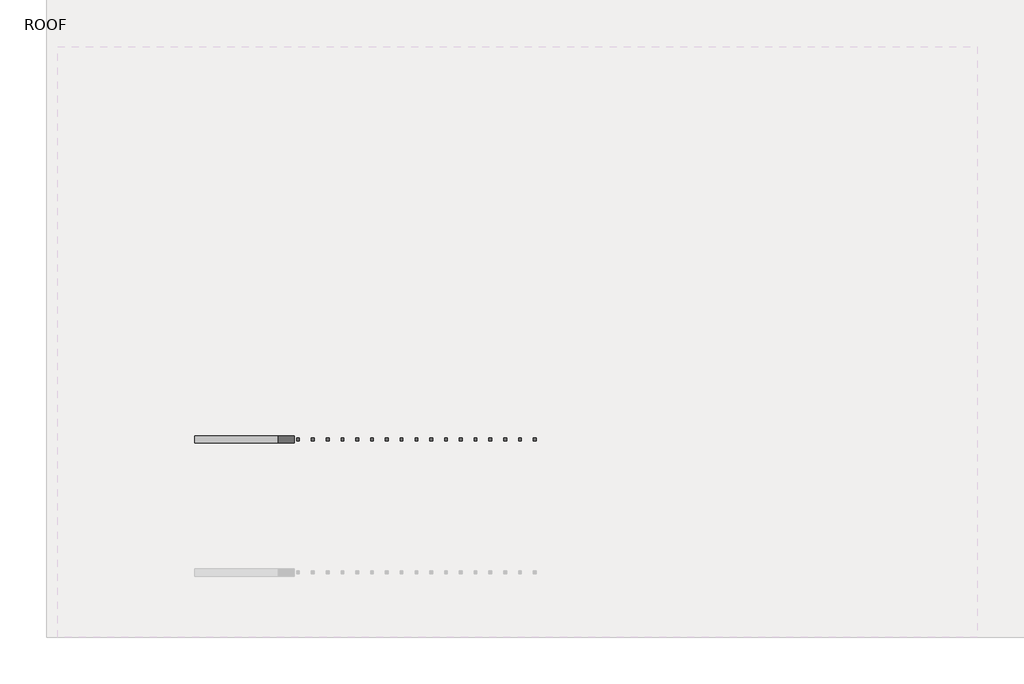
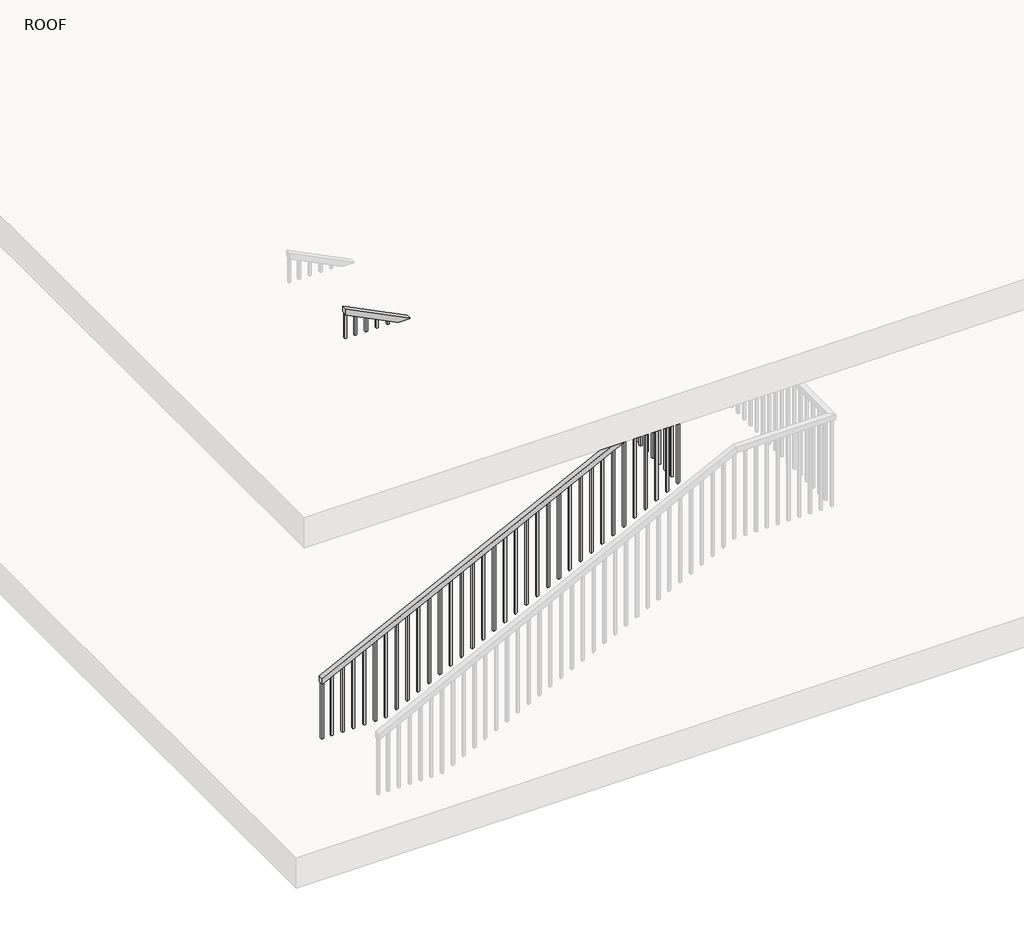
# One storey, part 2 of 2: 1 railing.
"""IFC4 building model written with IfcOpenShell, lengths in millimetres."""

from ifc_helpers import new_model, si_unit, frame, origin, place, context, project, spatial, polyline, outline, extrude, faceted_brep, element, save

model = new_model("IFC4")

# Units and contexts
model_context = context("Model", 3, world=origin())
ifc_project = project(units=[si_unit("LENGTHUNIT", "METRE", prefix="MILLI")], contexts=[model_context])

# Site, building, storey
site = spatial("IfcSite", under=ifc_project)
building = spatial("IfcBuilding", under=site)
storey = spatial("IfcBuildingStorey", under=building, Name="ROOF", Elevation=12192.0)

# Railing
placement = place(None, origin())
element("IfcRailing", 1, ObjectType="Handrail - Rectangular", at=placement, inside=storey, context=model_context, shape_type="SolidModel", body=[
    faceted_brep([(-8362.2800418, -4455.7090076, 13106.4), (-8362.2800418, -4455.7090076, 13049.6038734), (-8362.2800418, -4506.5090076, 13049.6038734), (-8362.2800418, -4506.5090076, 13106.4), (-5111.0800418, -4455.7090076, 14732.0), (-5060.2800418, -4455.7090076, 14700.6038734), (-5060.2800418, -4506.5090076, 14700.6038734), (-5111.0800418, -4506.5090076, 14732.0), (-5111.0800418, -4455.7090076, 14782.8), (-5060.2800418, -4455.7090076, 14732.0), (-5060.2800418, -4506.5090076, 14732.0), (-5111.0800418, -4506.5090076, 14782.8), (-5034.8800418, -4455.7090076, 14782.8), (-5034.8800418, -4455.7090076, 14732.0), (-4984.0800418, -4506.5090076, 14732.0), (-4984.0800418, -4506.5090076, 14782.8), (-5034.8800418, -4379.5090076, 14782.8), (-5034.8800418, -4379.5090076, 14732.0), (-4984.0800418, -4379.5090076, 14732.0), (-4984.0800418, -4379.5090076, 14782.8), (-5034.8800418, -3907.7346494, 14782.8), (-5034.8800418, -3856.9346494, 14732.0), (-4984.0800418, -3856.9346494, 14732.0), (-4984.0800418, -3907.7346494, 14782.8), (-5034.8800418, -3907.7346494, 14833.6), (-5034.8800418, -3856.9346494, 14782.8), (-4984.0800418, -3856.9346494, 14782.8), (-4984.0800418, -3907.7346494, 14833.6), (-5034.8800418, -3831.5346494, 14833.6), (-5034.8800418, -3831.5346494, 14782.8), (-4984.0800418, -3780.7346494, 14782.8), (-4984.0800418, -3780.7346494, 14833.6), (-5111.0800418, -3831.5346494, 14833.6), (-5123.072295, -3831.5346494, 14782.8), (-5123.072295, -3780.7346494, 14782.8), (-5111.0800418, -3780.7346494, 14833.6), (-7752.6800418, -3831.5346494, 16154.4), (-7752.6800418, -3780.7346494, 16154.4), (-7752.6800418, -3780.7346494, 16097.6038734), (-7752.6800418, -3831.5346494, 16097.6038734)], [[[0, 1, 2, 3]], [[1, 0, 4, 5]], [[2, 1, 5, 6]], [[3, 2, 6, 7]], [[0, 3, 7, 4]], [[5, 4, 8, 9]], [[6, 5, 9, 10]], [[7, 6, 10, 11]], [[4, 7, 11, 8]], [[9, 8, 12, 13]], [[10, 9, 13, 14]], [[11, 10, 14, 15]], [[8, 11, 15, 12]], [[13, 12, 16, 17]], [[14, 13, 17, 18]], [[15, 14, 18, 19]], [[12, 15, 19, 16]], [[17, 16, 20, 21]], [[18, 17, 21, 22]], [[19, 18, 22, 23]], [[16, 19, 23, 20]], [[21, 20, 24, 25]], [[22, 21, 25, 26]], [[23, 22, 26, 27]], [[20, 23, 27, 24]], [[25, 24, 28, 29]], [[26, 25, 29, 30]], [[27, 26, 30, 31]], [[24, 27, 31, 28]], [[29, 28, 32, 33]], [[30, 29, 33, 34]], [[31, 30, 34, 35]], [[28, 31, 35, 32]], [[36, 37, 38, 39]], [[33, 32, 36, 39]], [[34, 33, 39, 38]], [[35, 34, 38, 37]], [[32, 35, 37, 36]]]),
    extrude(outline(polyline([(16042.0413734, -7641.5550418), (16051.5663734, -7660.6050418), (15193.9625, -7660.6050418), (15184.4375, -7641.5550418), (16042.0413734, -7641.5550418)])), frame((0.0, -3815.6596494, 0.0), z_axis=(0.0, 1.0, 0.0), x_axis=(0.0, 0.0, 1.0)), (0.0, 0.0, 1.0), 19.05),
    extrude(outline(polyline([(15991.2413734, -7539.9550418), (16000.7663734, -7559.0050418), (15143.1625, -7559.0050418), (15133.6375, -7539.9550418), (15991.2413734, -7539.9550418)])), frame((0.0, -3815.6596494, 0.0), z_axis=(0.0, 1.0, 0.0), x_axis=(0.0, 0.0, 1.0)), (0.0, 0.0, 1.0), 19.05),
    extrude(outline(polyline([(15940.4413734, -7438.3550418), (15949.9663734, -7457.4050418), (15092.3625, -7457.4050418), (15082.8375, -7438.3550418), (15940.4413734, -7438.3550418)])), frame((0.0, -3815.6596494, 0.0), z_axis=(0.0, 1.0, 0.0), x_axis=(0.0, 0.0, 1.0)), (0.0, 0.0, 1.0), 19.05),
    extrude(outline(polyline([(15889.6413734, -7336.7550418), (15899.1663734, -7355.8050418), (15041.5625, -7355.8050418), (15032.0375, -7336.7550418), (15889.6413734, -7336.7550418)])), frame((0.0, -3815.6596494, 0.0), z_axis=(0.0, 1.0, 0.0), x_axis=(0.0, 0.0, 1.0)), (0.0, 0.0, 1.0), 19.05),
    extrude(outline(polyline([(15838.8413734, -7235.1550418), (15848.3663734, -7254.2050418), (14990.7625, -7254.2050418), (14981.2375, -7235.1550418), (15838.8413734, -7235.1550418)])), frame((0.0, -3815.6596494, 0.0), z_axis=(0.0, 1.0, 0.0), x_axis=(0.0, 0.0, 1.0)), (0.0, 0.0, 1.0), 19.05),
    extrude(outline(polyline([(15788.0413734, -7133.5550418), (15797.5663734, -7152.6050418), (14939.9625, -7152.6050418), (14930.4375, -7133.5550418), (15788.0413734, -7133.5550418)])), frame((0.0, -3815.6596494, 0.0), z_axis=(0.0, 1.0, 0.0), x_axis=(0.0, 0.0, 1.0)), (0.0, 0.0, 1.0), 19.05),
    extrude(outline(polyline([(15737.2413734, -7031.9550418), (15746.7663734, -7051.0050418), (14889.1625, -7051.0050418), (14879.6375, -7031.9550418), (15737.2413734, -7031.9550418)])), frame((0.0, -3815.6596494, 0.0), z_axis=(0.0, 1.0, 0.0), x_axis=(0.0, 0.0, 1.0)), (0.0, 0.0, 1.0), 19.05),
    extrude(outline(polyline([(15686.4413734, -6930.3550418), (15695.9663734, -6949.4050418), (14838.3625, -6949.4050418), (14828.8375, -6930.3550418), (15686.4413734, -6930.3550418)])), frame((0.0, -3815.6596494, 0.0), z_axis=(0.0, 1.0, 0.0), x_axis=(0.0, 0.0, 1.0)), (0.0, 0.0, 1.0), 19.05),
    extrude(outline(polyline([(15635.6413734, -6828.7550418), (15645.1663734, -6847.8050418), (14787.5625, -6847.8050418), (14778.0375, -6828.7550418), (15635.6413734, -6828.7550418)])), frame((0.0, -3815.6596494, 0.0), z_axis=(0.0, 1.0, 0.0), x_axis=(0.0, 0.0, 1.0)), (0.0, 0.0, 1.0), 19.05),
    extrude(outline(polyline([(15584.8413734, -6727.1550418), (15594.3663734, -6746.2050418), (14736.7625, -6746.2050418), (14727.2375, -6727.1550418), (15584.8413734, -6727.1550418)])), frame((0.0, -3815.6596494, 0.0), z_axis=(0.0, 1.0, 0.0), x_axis=(0.0, 0.0, 1.0)), (0.0, 0.0, 1.0), 19.05),
    extrude(outline(polyline([(15534.0413734, -6625.5550418), (15543.5663734, -6644.6050418), (14685.9625, -6644.6050418), (14676.4375, -6625.5550418), (15534.0413734, -6625.5550418)])), frame((0.0, -3815.6596494, 0.0), z_axis=(0.0, 1.0, 0.0), x_axis=(0.0, 0.0, 1.0)), (0.0, 0.0, 1.0), 19.05),
    extrude(outline(polyline([(15483.2413734, -6523.9550418), (15492.7663734, -6543.0050418), (14635.1625, -6543.0050418), (14625.6375, -6523.9550418), (15483.2413734, -6523.9550418)])), frame((0.0, -3815.6596494, 0.0), z_axis=(0.0, 1.0, 0.0), x_axis=(0.0, 0.0, 1.0)), (0.0, 0.0, 1.0), 19.05),
    extrude(outline(polyline([(15432.4413734, -6422.3550418), (15441.9663734, -6441.4050418), (14584.3625, -6441.4050418), (14574.8375, -6422.3550418), (15432.4413734, -6422.3550418)])), frame((0.0, -3815.6596494, 0.0), z_axis=(0.0, 1.0, 0.0), x_axis=(0.0, 0.0, 1.0)), (0.0, 0.0, 1.0), 19.05),
    extrude(outline(polyline([(15381.6413734, -6320.7550418), (15391.1663734, -6339.8050418), (14533.5625, -6339.8050418), (14524.0375, -6320.7550418), (15381.6413734, -6320.7550418)])), frame((0.0, -3815.6596494, 0.0), z_axis=(0.0, 1.0, 0.0), x_axis=(0.0, 0.0, 1.0)), (0.0, 0.0, 1.0), 19.05),
    extrude(outline(polyline([(15330.8413734, -6219.1550418), (15340.3663734, -6238.2050418), (14482.7625, -6238.2050418), (14473.2375, -6219.1550418), (15330.8413734, -6219.1550418)])), frame((0.0, -3815.6596494, 0.0), z_axis=(0.0, 1.0, 0.0), x_axis=(0.0, 0.0, 1.0)), (0.0, 0.0, 1.0), 19.05),
    extrude(outline(polyline([(15280.0413734, -6117.5550418), (15289.5663734, -6136.6050418), (14431.9625, -6136.6050418), (14422.4375, -6117.5550418), (15280.0413734, -6117.5550418)])), frame((0.0, -3815.6596494, 0.0), z_axis=(0.0, 1.0, 0.0), x_axis=(0.0, 0.0, 1.0)), (0.0, 0.0, 1.0), 19.05),
    extrude(outline(polyline([(15229.2413734, -6015.9550418), (15238.7663734, -6035.0050418), (14381.1625, -6035.0050418), (14371.6375, -6015.9550418), (15229.2413734, -6015.9550418)])), frame((0.0, -3815.6596494, 0.0), z_axis=(0.0, 1.0, 0.0), x_axis=(0.0, 0.0, 1.0)), (0.0, 0.0, 1.0), 19.05),
    extrude(outline(polyline([(15178.4413734, -5914.3550418), (15187.9663734, -5933.4050418), (14330.3625, -5933.4050418), (14320.8375, -5914.3550418), (15178.4413734, -5914.3550418)])), frame((0.0, -3815.6596494, 0.0), z_axis=(0.0, 1.0, 0.0), x_axis=(0.0, 0.0, 1.0)), (0.0, 0.0, 1.0), 19.05),
    extrude(outline(polyline([(15127.6413734, -5812.7550418), (15137.1663734, -5831.8050418), (14279.5625, -5831.8050418), (14270.0375, -5812.7550418), (15127.6413734, -5812.7550418)])), frame((0.0, -3815.6596494, 0.0), z_axis=(0.0, 1.0, 0.0), x_axis=(0.0, 0.0, 1.0)), (0.0, 0.0, 1.0), 19.05),
    extrude(outline(polyline([(15076.8413734, -5711.1550418), (15086.3663734, -5730.2050418), (14228.7625, -5730.2050418), (14219.2375, -5711.1550418), (15076.8413734, -5711.1550418)])), frame((0.0, -3815.6596494, 0.0), z_axis=(0.0, 1.0, 0.0), x_axis=(0.0, 0.0, 1.0)), (0.0, 0.0, 1.0), 19.05),
    extrude(outline(polyline([(15026.0413734, -5609.5550418), (15035.5663734, -5628.6050418), (14177.9625, -5628.6050418), (14168.4375, -5609.5550418), (15026.0413734, -5609.5550418)])), frame((0.0, -3815.6596494, 0.0), z_axis=(0.0, 1.0, 0.0), x_axis=(0.0, 0.0, 1.0)), (0.0, 0.0, 1.0), 19.05),
    extrude(outline(polyline([(14975.2413734, -5507.9550418), (14984.7663734, -5527.0050418), (14127.1625, -5527.0050418), (14117.6375, -5507.9550418), (14975.2413734, -5507.9550418)])), frame((0.0, -3815.6596494, 0.0), z_axis=(0.0, 1.0, 0.0), x_axis=(0.0, 0.0, 1.0)), (0.0, 0.0, 1.0), 19.05),
    extrude(outline(polyline([(14924.4413734, -5406.3550418), (14933.9663734, -5425.4050418), (14076.3625, -5425.4050418), (14066.8375, -5406.3550418), (14924.4413734, -5406.3550418)])), frame((0.0, -3815.6596494, 0.0), z_axis=(0.0, 1.0, 0.0), x_axis=(0.0, 0.0, 1.0)), (0.0, 0.0, 1.0), 19.05),
    extrude(outline(polyline([(14873.6413734, -5304.7550418), (14883.1663734, -5323.8050418), (14025.5625, -5323.8050418), (14016.0375, -5304.7550418), (14873.6413734, -5304.7550418)])), frame((0.0, -3815.6596494, 0.0), z_axis=(0.0, 1.0, 0.0), x_axis=(0.0, 0.0, 1.0)), (0.0, 0.0, 1.0), 19.05),
    extrude(outline(polyline([(14822.8413734, -5203.1550418), (14832.3663734, -5222.2050418), (13974.7625, -5222.2050418), (13965.2375, -5203.1550418), (14822.8413734, -5203.1550418)])), frame((0.0, -3815.6596494, 0.0), z_axis=(0.0, 1.0, 0.0), x_axis=(0.0, 0.0, 1.0)), (0.0, 0.0, 1.0), 19.05),
    extrude(outline(polyline([(14782.8, -5101.5550418), (14782.8, -5120.6050418), (13923.9625, -5120.6050418), (13914.4375, -5101.5550418), (14782.8, -5101.5550418)])), frame((0.0, -3815.6596494, 0.0), z_axis=(0.0, 1.0, 0.0), x_axis=(0.0, 0.0, 1.0)), (0.0, 0.0, 1.0), 19.05),
    extrude(outline(polyline([(-4999.9550418, -3881.0340076), (-5019.0050418, -3881.0340076), (-5019.0050418, -3861.9840076), (-4999.9550418, -3861.9840076), (-4999.9550418, -3881.0340076)])), frame((0.0, 0.0, 13868.4), z_axis=(0.0, 0.0, 1.0), x_axis=(1.0, 0.0, 0.0)), (0.0, 0.0, 1.0), 863.6),
    extrude(outline(polyline([(-4999.9550418, -3982.6340076), (-5019.0050418, -3982.6340076), (-5019.0050418, -3963.5840076), (-4999.9550418, -3963.5840076), (-4999.9550418, -3982.6340076)])), frame((0.0, 0.0, 13868.4), z_axis=(0.0, 0.0, 1.0), x_axis=(1.0, 0.0, 0.0)), (0.0, 0.0, 1.0), 863.6),
    extrude(outline(polyline([(-4999.9550418, -4084.2340076), (-5019.0050418, -4084.2340076), (-5019.0050418, -4065.1840076), (-4999.9550418, -4065.1840076), (-4999.9550418, -4084.2340076)])), frame((0.0, 0.0, 13868.4), z_axis=(0.0, 0.0, 1.0), x_axis=(1.0, 0.0, 0.0)), (0.0, 0.0, 1.0), 863.6),
    extrude(outline(polyline([(-4999.9550418, -4185.8340076), (-5019.0050418, -4185.8340076), (-5019.0050418, -4166.7840076), (-4999.9550418, -4166.7840076), (-4999.9550418, -4185.8340076)])), frame((0.0, 0.0, 13868.4), z_axis=(0.0, 0.0, 1.0), x_axis=(1.0, 0.0, 0.0)), (0.0, 0.0, 1.0), 863.6),
    extrude(outline(polyline([(-4999.9550418, -4287.4340076), (-5019.0050418, -4287.4340076), (-5019.0050418, -4268.3840076), (-4999.9550418, -4268.3840076), (-4999.9550418, -4287.4340076)])), frame((0.0, 0.0, 13868.4), z_axis=(0.0, 0.0, 1.0), x_axis=(1.0, 0.0, 0.0)), (0.0, 0.0, 1.0), 863.6),
    extrude(outline(polyline([(-4999.9550418, -4389.0340076), (-5019.0050418, -4389.0340076), (-5019.0050418, -4369.9840076), (-4999.9550418, -4369.9840076), (-4999.9550418, -4389.0340076)])), frame((0.0, 0.0, 13868.4), z_axis=(0.0, 0.0, 1.0), x_axis=(1.0, 0.0, 0.0)), (0.0, 0.0, 1.0), 863.6),
    extrude(outline(polyline([(14679.9663734, -5101.5550418), (14670.4413734, -5120.6050418), (13812.8375, -5120.6050418), (13822.3625, -5101.5550418), (14679.9663734, -5101.5550418)])), frame((0.0, -4490.6340076, 0.0), z_axis=(0.0, 1.0, 0.0), x_axis=(0.0, 0.0, 1.0)), (0.0, 0.0, 1.0), 19.05),
    extrude(outline(polyline([(14629.1663734, -5203.1550418), (14619.6413734, -5222.2050418), (13762.0375, -5222.2050418), (13771.5625, -5203.1550418), (14629.1663734, -5203.1550418)])), frame((0.0, -4490.6340076, 0.0), z_axis=(0.0, 1.0, 0.0), x_axis=(0.0, 0.0, 1.0)), (0.0, 0.0, 1.0), 19.05),
    extrude(outline(polyline([(14578.3663734, -5304.7550418), (14568.8413734, -5323.8050418), (13711.2375, -5323.8050418), (13720.7625, -5304.7550418), (14578.3663734, -5304.7550418)])), frame((0.0, -4490.6340076, 0.0), z_axis=(0.0, 1.0, 0.0), x_axis=(0.0, 0.0, 1.0)), (0.0, 0.0, 1.0), 19.05),
    extrude(outline(polyline([(14527.5663734, -5406.3550418), (14518.0413734, -5425.4050418), (13660.4375, -5425.4050418), (13669.9625, -5406.3550418), (14527.5663734, -5406.3550418)])), frame((0.0, -4490.6340076, 0.0), z_axis=(0.0, 1.0, 0.0), x_axis=(0.0, 0.0, 1.0)), (0.0, 0.0, 1.0), 19.05),
    extrude(outline(polyline([(14476.7663734, -5507.9550418), (14467.2413734, -5527.0050418), (13609.6375, -5527.0050418), (13619.1625, -5507.9550418), (14476.7663734, -5507.9550418)])), frame((0.0, -4490.6340076, 0.0), z_axis=(0.0, 1.0, 0.0), x_axis=(0.0, 0.0, 1.0)), (0.0, 0.0, 1.0), 19.05),
    extrude(outline(polyline([(14425.9663734, -5609.5550418), (14416.4413734, -5628.6050418), (13558.8375, -5628.6050418), (13568.3625, -5609.5550418), (14425.9663734, -5609.5550418)])), frame((0.0, -4490.6340076, 0.0), z_axis=(0.0, 1.0, 0.0), x_axis=(0.0, 0.0, 1.0)), (0.0, 0.0, 1.0), 19.05),
    extrude(outline(polyline([(14375.1663734, -5711.1550418), (14365.6413734, -5730.2050418), (13508.0375, -5730.2050418), (13517.5625, -5711.1550418), (14375.1663734, -5711.1550418)])), frame((0.0, -4490.6340076, 0.0), z_axis=(0.0, 1.0, 0.0), x_axis=(0.0, 0.0, 1.0)), (0.0, 0.0, 1.0), 19.05),
    extrude(outline(polyline([(14324.3663734, -5812.7550418), (14314.8413734, -5831.8050418), (13457.2375, -5831.8050418), (13466.7625, -5812.7550418), (14324.3663734, -5812.7550418)])), frame((0.0, -4490.6340076, 0.0), z_axis=(0.0, 1.0, 0.0), x_axis=(0.0, 0.0, 1.0)), (0.0, 0.0, 1.0), 19.05),
    extrude(outline(polyline([(14273.5663734, -5914.3550418), (14264.0413734, -5933.4050418), (13406.4375, -5933.4050418), (13415.9625, -5914.3550418), (14273.5663734, -5914.3550418)])), frame((0.0, -4490.6340076, 0.0), z_axis=(0.0, 1.0, 0.0), x_axis=(0.0, 0.0, 1.0)), (0.0, 0.0, 1.0), 19.05),
    extrude(outline(polyline([(14222.7663734, -6015.9550418), (14213.2413734, -6035.0050418), (13355.6375, -6035.0050418), (13365.1625, -6015.9550418), (14222.7663734, -6015.9550418)])), frame((0.0, -4490.6340076, 0.0), z_axis=(0.0, 1.0, 0.0), x_axis=(0.0, 0.0, 1.0)), (0.0, 0.0, 1.0), 19.05),
    extrude(outline(polyline([(14171.9663734, -6117.5550418), (14162.4413734, -6136.6050418), (13304.8375, -6136.6050418), (13314.3625, -6117.5550418), (14171.9663734, -6117.5550418)])), frame((0.0, -4490.6340076, 0.0), z_axis=(0.0, 1.0, 0.0), x_axis=(0.0, 0.0, 1.0)), (0.0, 0.0, 1.0), 19.05),
    extrude(outline(polyline([(14121.1663734, -6219.1550418), (14111.6413734, -6238.2050418), (13254.0375, -6238.2050418), (13263.5625, -6219.1550418), (14121.1663734, -6219.1550418)])), frame((0.0, -4490.6340076, 0.0), z_axis=(0.0, 1.0, 0.0), x_axis=(0.0, 0.0, 1.0)), (0.0, 0.0, 1.0), 19.05),
    extrude(outline(polyline([(14070.3663734, -6320.7550418), (14060.8413734, -6339.8050418), (13203.2375, -6339.8050418), (13212.7625, -6320.7550418), (14070.3663734, -6320.7550418)])), frame((0.0, -4490.6340076, 0.0), z_axis=(0.0, 1.0, 0.0), x_axis=(0.0, 0.0, 1.0)), (0.0, 0.0, 1.0), 19.05),
    extrude(outline(polyline([(14019.5663734, -6422.3550418), (14010.0413734, -6441.4050418), (13152.4375, -6441.4050418), (13161.9625, -6422.3550418), (14019.5663734, -6422.3550418)])), frame((0.0, -4490.6340076, 0.0), z_axis=(0.0, 1.0, 0.0), x_axis=(0.0, 0.0, 1.0)), (0.0, 0.0, 1.0), 19.05),
    extrude(outline(polyline([(13968.7663734, -6523.9550418), (13959.2413734, -6543.0050418), (13101.6375, -6543.0050418), (13111.1625, -6523.9550418), (13968.7663734, -6523.9550418)])), frame((0.0, -4490.6340076, 0.0), z_axis=(0.0, 1.0, 0.0), x_axis=(0.0, 0.0, 1.0)), (0.0, 0.0, 1.0), 19.05),
    extrude(outline(polyline([(13917.9663734, -6625.5550418), (13908.4413734, -6644.6050418), (13050.8375, -6644.6050418), (13060.3625, -6625.5550418), (13917.9663734, -6625.5550418)])), frame((0.0, -4490.6340076, 0.0), z_axis=(0.0, 1.0, 0.0), x_axis=(0.0, 0.0, 1.0)), (0.0, 0.0, 1.0), 19.05),
    extrude(outline(polyline([(13867.1663734, -6727.1550418), (13857.6413734, -6746.2050418), (13000.0375, -6746.2050418), (13009.5625, -6727.1550418), (13867.1663734, -6727.1550418)])), frame((0.0, -4490.6340076, 0.0), z_axis=(0.0, 1.0, 0.0), x_axis=(0.0, 0.0, 1.0)), (0.0, 0.0, 1.0), 19.05),
    extrude(outline(polyline([(13816.3663734, -6828.7550418), (13806.8413734, -6847.8050418), (12949.2375, -6847.8050418), (12958.7625, -6828.7550418), (13816.3663734, -6828.7550418)])), frame((0.0, -4490.6340076, 0.0), z_axis=(0.0, 1.0, 0.0), x_axis=(0.0, 0.0, 1.0)), (0.0, 0.0, 1.0), 19.05),
    extrude(outline(polyline([(13765.5663734, -6930.3550418), (13756.0413734, -6949.4050418), (12898.4375, -6949.4050418), (12907.9625, -6930.3550418), (13765.5663734, -6930.3550418)])), frame((0.0, -4490.6340076, 0.0), z_axis=(0.0, 1.0, 0.0), x_axis=(0.0, 0.0, 1.0)), (0.0, 0.0, 1.0), 19.05),
    extrude(outline(polyline([(13714.7663734, -7031.9550418), (13705.2413734, -7051.0050418), (12847.6375, -7051.0050418), (12857.1625, -7031.9550418), (13714.7663734, -7031.9550418)])), frame((0.0, -4490.6340076, 0.0), z_axis=(0.0, 1.0, 0.0), x_axis=(0.0, 0.0, 1.0)), (0.0, 0.0, 1.0), 19.05),
    extrude(outline(polyline([(13663.9663734, -7133.5550418), (13654.4413734, -7152.6050418), (12796.8375, -7152.6050418), (12806.3625, -7133.5550418), (13663.9663734, -7133.5550418)])), frame((0.0, -4490.6340076, 0.0), z_axis=(0.0, 1.0, 0.0), x_axis=(0.0, 0.0, 1.0)), (0.0, 0.0, 1.0), 19.05),
    extrude(outline(polyline([(13613.1663734, -7235.1550418), (13603.6413734, -7254.2050418), (12746.0375, -7254.2050418), (12755.5625, -7235.1550418), (13613.1663734, -7235.1550418)])), frame((0.0, -4490.6340076, 0.0), z_axis=(0.0, 1.0, 0.0), x_axis=(0.0, 0.0, 1.0)), (0.0, 0.0, 1.0), 19.05),
    extrude(outline(polyline([(13562.3663734, -7336.7550418), (13552.8413734, -7355.8050418), (12695.2375, -7355.8050418), (12704.7625, -7336.7550418), (13562.3663734, -7336.7550418)])), frame((0.0, -4490.6340076, 0.0), z_axis=(0.0, 1.0, 0.0), x_axis=(0.0, 0.0, 1.0)), (0.0, 0.0, 1.0), 19.05),
    extrude(outline(polyline([(13511.5663734, -7438.3550418), (13502.0413734, -7457.4050418), (12644.4375, -7457.4050418), (12653.9625, -7438.3550418), (13511.5663734, -7438.3550418)])), frame((0.0, -4490.6340076, 0.0), z_axis=(0.0, 1.0, 0.0), x_axis=(0.0, 0.0, 1.0)), (0.0, 0.0, 1.0), 19.05),
    extrude(outline(polyline([(13460.7663734, -7539.9550418), (13451.2413734, -7559.0050418), (12593.6375, -7559.0050418), (12603.1625, -7539.9550418), (13460.7663734, -7539.9550418)])), frame((0.0, -4490.6340076, 0.0), z_axis=(0.0, 1.0, 0.0), x_axis=(0.0, 0.0, 1.0)), (0.0, 0.0, 1.0), 19.05),
    extrude(outline(polyline([(13409.9663734, -7641.5550418), (13400.4413734, -7660.6050418), (12542.8375, -7660.6050418), (12552.3625, -7641.5550418), (13409.9663734, -7641.5550418)])), frame((0.0, -4490.6340076, 0.0), z_axis=(0.0, 1.0, 0.0), x_axis=(0.0, 0.0, 1.0)), (0.0, 0.0, 1.0), 19.05),
    extrude(outline(polyline([(13359.1663734, -7743.1550418), (13349.6413734, -7762.2050418), (12492.0375, -7762.2050418), (12501.5625, -7743.1550418), (13359.1663734, -7743.1550418)])), frame((0.0, -4490.6340076, 0.0), z_axis=(0.0, 1.0, 0.0), x_axis=(0.0, 0.0, 1.0)), (0.0, 0.0, 1.0), 19.05),
    extrude(outline(polyline([(13308.3663734, -7844.7550418), (13298.8413734, -7863.8050418), (12441.2375, -7863.8050418), (12450.7625, -7844.7550418), (13308.3663734, -7844.7550418)])), frame((0.0, -4490.6340076, 0.0), z_axis=(0.0, 1.0, 0.0), x_axis=(0.0, 0.0, 1.0)), (0.0, 0.0, 1.0), 19.05),
    extrude(outline(polyline([(13257.5663734, -7946.3550418), (13248.0413734, -7965.4050418), (12390.4375, -7965.4050418), (12399.9625, -7946.3550418), (13257.5663734, -7946.3550418)])), frame((0.0, -4490.6340076, 0.0), z_axis=(0.0, 1.0, 0.0), x_axis=(0.0, 0.0, 1.0)), (0.0, 0.0, 1.0), 19.05),
    extrude(outline(polyline([(13206.7663734, -8047.9550418), (13197.2413734, -8067.0050418), (12339.6375, -8067.0050418), (12349.1625, -8047.9550418), (13206.7663734, -8047.9550418)])), frame((0.0, -4490.6340076, 0.0), z_axis=(0.0, 1.0, 0.0), x_axis=(0.0, 0.0, 1.0)), (0.0, 0.0, 1.0), 19.05),
    extrude(outline(polyline([(13155.9663734, -8149.5550418), (13146.4413734, -8168.6050418), (12288.8375, -8168.6050418), (12298.3625, -8149.5550418), (13155.9663734, -8149.5550418)])), frame((0.0, -4490.6340076, 0.0), z_axis=(0.0, 1.0, 0.0), x_axis=(0.0, 0.0, 1.0)), (0.0, 0.0, 1.0), 19.05),
    extrude(outline(polyline([(13105.1663734, -8251.1550418), (13095.6413734, -8270.2050418), (12238.0375, -8270.2050418), (12247.5625, -8251.1550418), (13105.1663734, -8251.1550418)])), frame((0.0, -4490.6340076, 0.0), z_axis=(0.0, 1.0, 0.0), x_axis=(0.0, 0.0, 1.0)), (0.0, 0.0, 1.0), 19.05),
    extrude(outline(polyline([(-4999.9550418, -3815.6596494), (-5019.0050418, -3815.6596494), (-5019.0050418, -3796.6096494), (-4999.9550418, -3796.6096494), (-4999.9550418, -3815.6596494)])), frame((0.0, 0.0, 13868.4), z_axis=(0.0, 0.0, 1.0), x_axis=(1.0, 0.0, 0.0)), (0.0, 0.0, 1.0), 914.4),
    extrude(outline(polyline([(14732.0, -4999.9550418), (14732.0, -5019.0050418), (13863.6375, -5019.0050418), (13873.1625, -4999.9550418), (14732.0, -4999.9550418)])), frame((0.0, -4490.6340076, 0.0), z_axis=(0.0, 1.0, 0.0), x_axis=(0.0, 0.0, 1.0)), (0.0, 0.0, 1.0), 19.05),
    extrude(outline(polyline([(16088.0788734, -7733.6300418), (16097.6038734, -7752.6800418), (15240.0, -7752.6800418), (15230.475, -7733.6300418), (16088.0788734, -7733.6300418)])), frame((0.0, -3815.6596494, 0.0), z_axis=(0.0, 1.0, 0.0), x_axis=(0.0, 0.0, 1.0)), (0.0, 0.0, 1.0), 19.05),
    extrude(outline(polyline([(13059.1288734, -8343.2300418), (13049.6038734, -8362.2800418), (12192.0, -8362.2800418), (12201.525, -8343.2300418), (13059.1288734, -8343.2300418)])), frame((0.0, -4490.6340076, 0.0), z_axis=(0.0, 1.0, 0.0), x_axis=(0.0, 0.0, 1.0)), (0.0, 0.0, 1.0), 19.05),
])

save(model, "model.ifc")

# Revit data of these elements
# Type "Handrail - Rectangular"
#   Assembly Code = "C2010400"
#   built-in parameter 1008612 = 0.0416667 (stored number, unit not read)
#   built-in parameter 1008611 = 0.0416667 (stored number, unit not read)
#   built-in parameter 1008609 = 0.333333 (stored number, unit not read)
#   built-in parameter 1008604 = 0.166667 (stored number, unit not read)
#   built-in parameter 1008603 = 0.166667 (stored number, unit not read)
#   Railing Height = 3' - 0"
#   built-in parameter 1008630 = 2
#   built-in parameter 1008610 = 2
#   built-in parameter 1008618 = Baluster - Square : 3/4"
# Element 1 (IfcRailing, "Handrail - Rectangular")
#   Phase Created = New Construction
